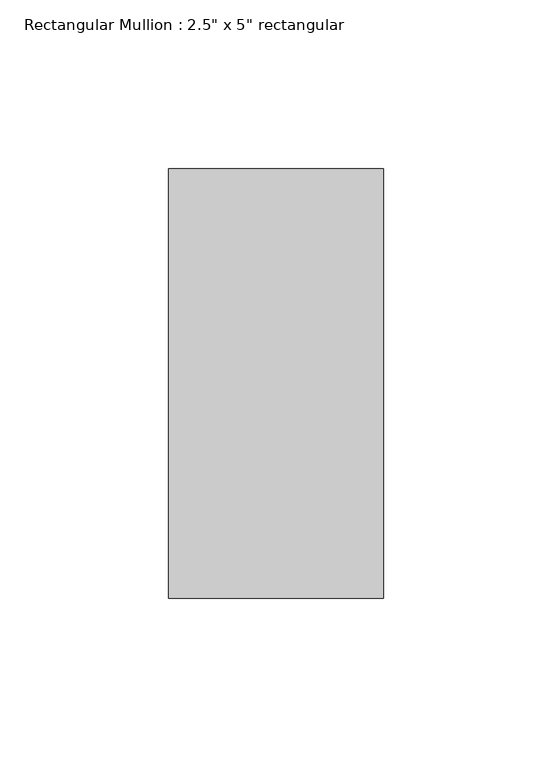
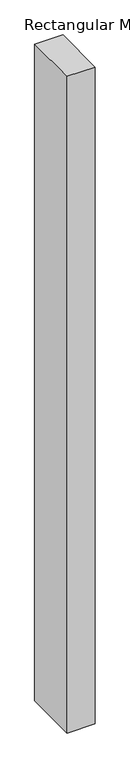
"""IFC4 building model written with IfcOpenShell, lengths in millimetres: member geometry."""

from ifc_helpers import new_model, si_unit, frame, origin, place, context, project, spatial, polyline, outline, extrude, source, transform, mapped, element, save


def member_3cfa9974(model_context):
    return source(origin(), model_context, "Body", "SweptSolid", [
        extrude(outline(polyline([(31.75, 63.5), (31.75, -63.5), (-31.75, -63.5), (-31.75, 63.5), (31.75, 63.5)])), frame((0.0, 0.0, -1569.0265415), z_axis=(0.0, 0.0, 1.0), x_axis=(1.0, 0.0, 0.0)), (0.0, 0.0, 1.0), 1569.0265415),
    ])


if __name__ == "__main__":
    model = new_model("IFC4")
    model_context = context("Model", 3, world=origin())
    ifc_project = project(units=[si_unit("LENGTHUNIT", "METRE", prefix="MILLI")], contexts=[model_context])
    site = spatial("IfcSite", under=ifc_project)
    building = spatial("IfcBuilding", under=site)
    placement = place(None, origin())
    member_shape = member_3cfa9974(model_context)
    element("IfcMember", 1, ObjectType="Rectangular Mullion : 2.5\" x 5\" rectangular", at=placement, inside=building, context=model_context, shape_type="MappedRepresentation", body=[
        mapped(member_shape, transform((0.0, 0.0, 0.0), x_axis=(1.0, 0.0, 0.0), y_axis=(0.0, 1.0, 0.0), z_axis=(0.0, 0.0, 1.0))),
    ])
    save(model, "model.ifc")

# Revit data of these elements
# Type "Rectangular Mullion : 2.5\" x 5\" rectangular"
#   built-in parameter 1007304 = 0.416667 (stored number, unit not read)
#   built-in parameter 1007301 = 0.104167 (stored number, unit not read)
#   built-in parameter 1007300 = 0.104167 (stored number, unit not read)
# Element 1 (IfcMember, "Rectangular Mullion : 2.5\" x 5\" rectangular")
#   Materials on its faces: "Aluminum"
# Materials
#   "Aluminum": class "Metal", colour RGB 247 247 247, transparency 0, Description = "Aluminum 6061", Cost = 0
